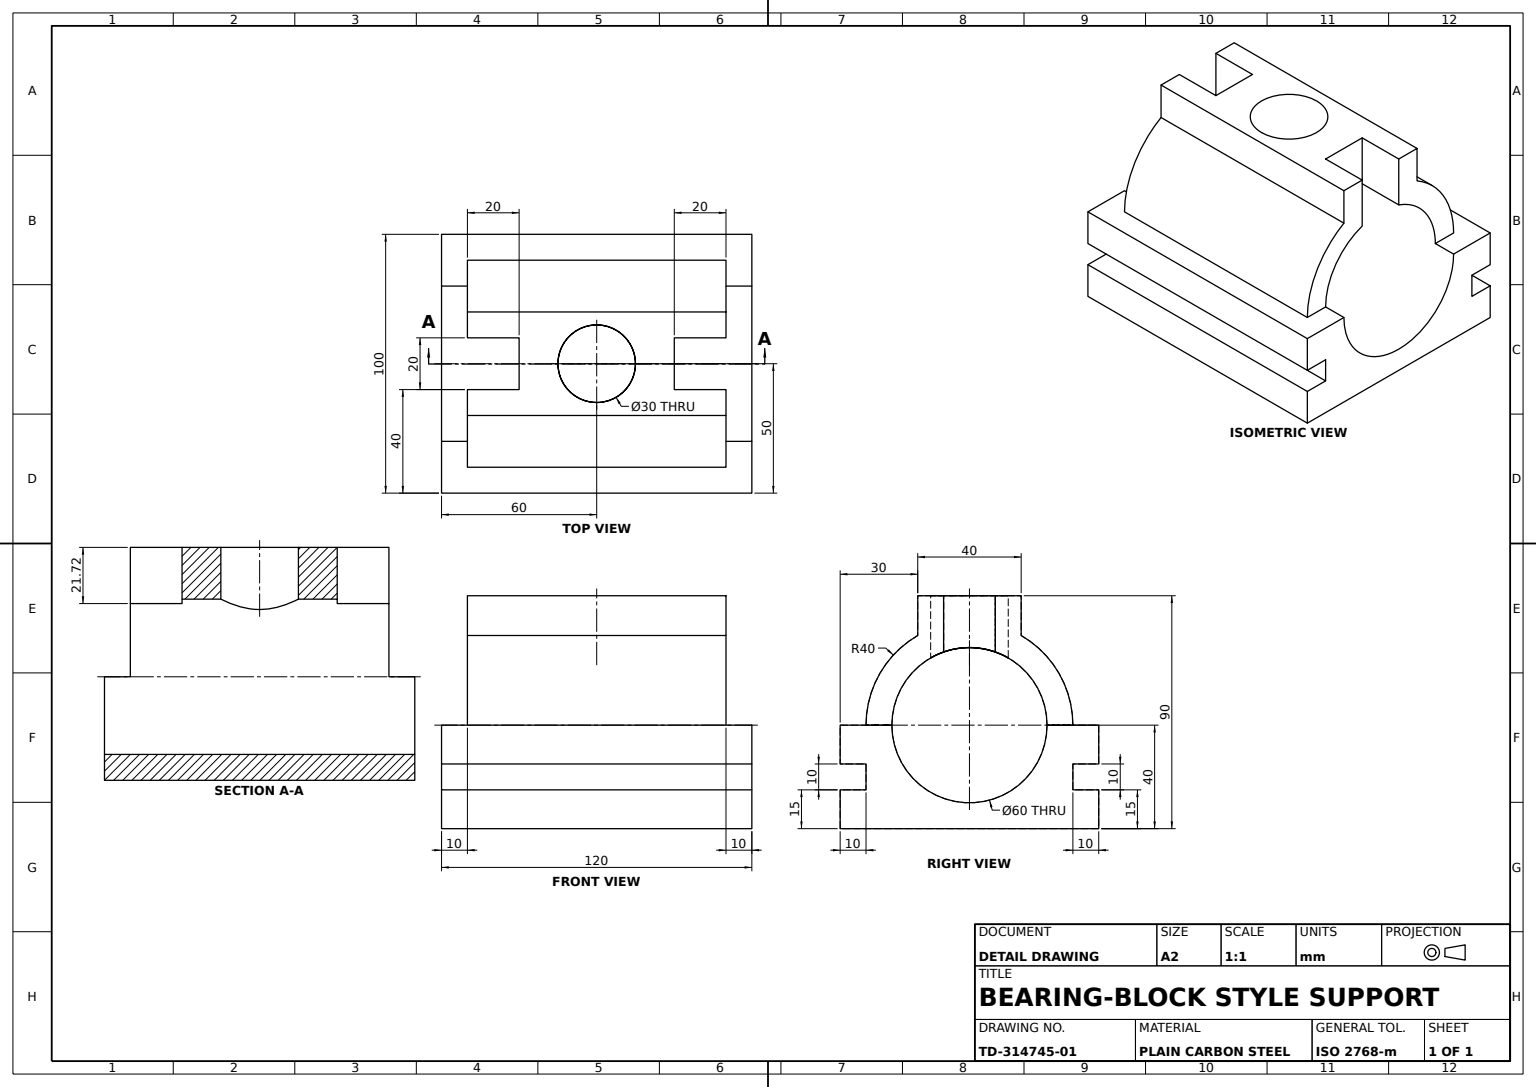
SolidWorks part; units mm, degrees
material "Plain Carbon Steel"
ref_plane "Front Plane" through (0, 0, 0) normal (0, 0, 1) x (1, 0, 0)
ref_plane "Top Plane" through (0, 0, 0) normal (0, 1, 0) x (1, 0, 0)
ref_plane "Right Plane" through (0, 0, 0) normal (1, 0, 0) x (0, 0, -1)
sketch "Base Profile Sketch" plane through (0, 0, 0) normal (0, 0, 1) x (1, 0, 0)
  line L0 (0, 0) -> (100, 0)
  line L1 (100, 0) -> (100, 15)
  line L2 (100, 15) -> (90, 15)
  line L3 (90, 15) -> (90, 25)
  line L4 (90, 25) -> (100, 25)
  line L5 (100, 25) -> (100, 40)
  line L6 (100, 40) -> (80, 40)
  line L7 (0, 40) -> (0, 25)
  line L8 (0, 25) -> (10, 25)
  line L9 (10, 25) -> (10, 15)
  line L10 (10, 15) -> (0, 15)
  line L11 (0, 15) -> (0, 0)
  line L12 (20, 40) -> (0, 40)
  arc A0 (20, 40) -> (80, 40) centre (50, 40) ccw
  dimension "D10" = 60
  dimension "D1" = 100
  dimension "D2" = 15
  dimension "D3" = 10
  dimension "D4" = 10
  dimension "D5" = 15
  dimension "D6" = 10
  dimension "D7" = 10
  dimension "D8" = 10
  dimension "D9" = 15
  dimension "D11" = 40
  dimension "D12" = 50
extrude "Base Block" add sketch "Base Profile Sketch" against normal blind 120
ref_plane "Housing Offset Plane" through (0, 0, -10) normal (0, 0, 1) x (1, 0, 0)
sketch "Bearing Housing Profile Sketch" plane through (0, 0, -10) normal (0, 0, 1) x (1, 0, 0)
  line L0 (10, 40) -> (20, 40)
  line L1 (30, 90) -> (70, 90)
  line L2 (30, 90) -> (30, 74.641)
  line L4 (70, 90) -> (70, 74.641)
  line L5 (80, 40) -> (90, 40)
  arc A0 (90, 40) -> (10, 40) centre (50, 40) ccw
  circle A1 centre (50, 40) radius 30
  dimension "D5" = 80
  dimension "D6" = 60
  dimension "D1" = 40
  dimension "D2" = 15.359
  dimension "D3" = 90
extrude "Bearing Housing" add sketch "Bearing Housing Profile Sketch" against normal blind 100 contours A1 L5 A0 L0 | A0 L4 L1 L2
sketch "Top Slots Sketch" plane through (0, 90, 0) normal (0, 1, 0) x (1, 0, 0)
  line L0 (30, 10) -> (70, 10) construction
  line L1 (40, 10) -> (60, 10)
  line L2 (40, 10) -> (40, 30)
  line L3 (40, 30) -> (60, 30)
  line L4 (60, 10) -> (60, 30)
  line L5 (30, 110) -> (70, 110) construction
  line L6 (40, 110) -> (60, 110)
  line L7 (40, 110) -> (40, 90)
  line L8 (40, 90) -> (60, 90)
  line L9 (60, 110) -> (60, 90)
  dimension "D1" = 20
  dimension "D2" = 40
  dimension "D3" = 20
  dimension "D4" = 20
  dimension "D5" = 40
  dimension "D6" = 20
extrude "Top Slots" cut sketch "Top Slots Sketch" against normal blind 30
sketch "Top Hole Sketch" plane through (0, 90, 0) normal (0, 1, 0) x (1, 0, 0)
  circle A0 centre (50, 60) radius 15
  dimension "D1" = 30
  dimension "D2" = 50
  dimension "D3" = 30
extrude "Top Hole Ø30" cut sketch "Top Hole Sketch" against normal blind 30
